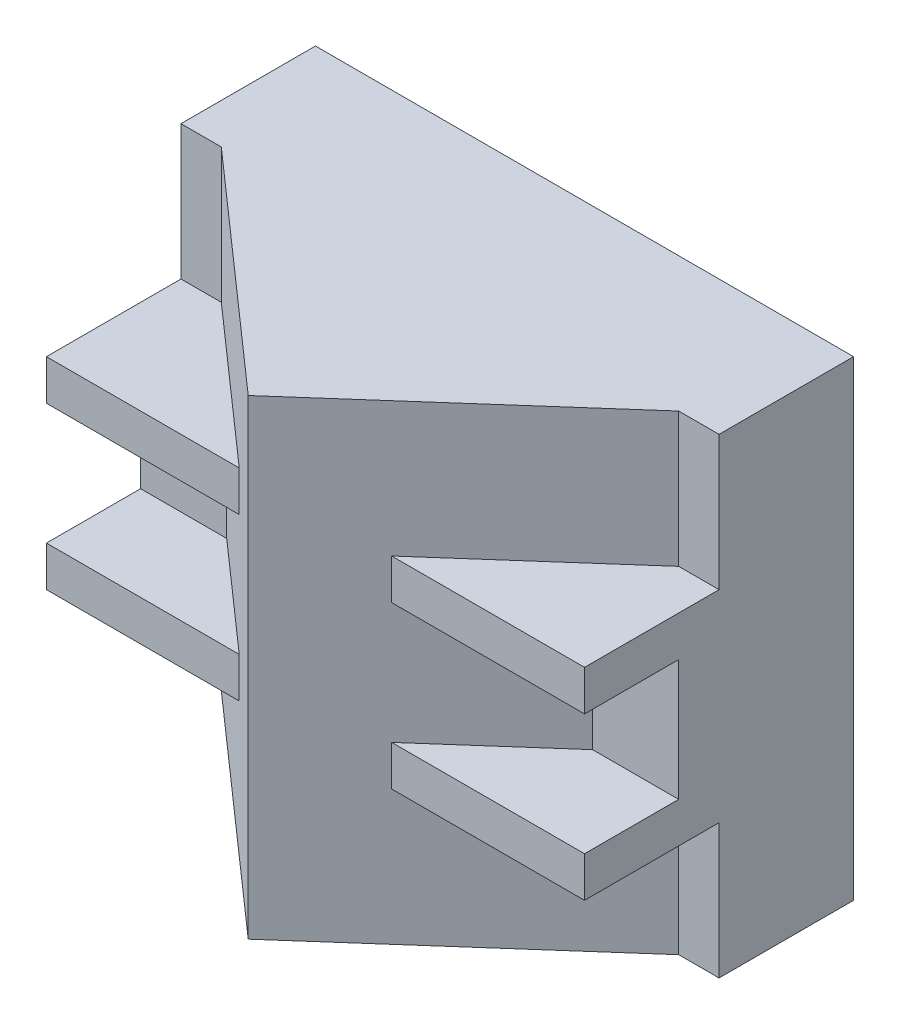
ISO-10303-21;
HEADER;
FILE_DESCRIPTION(('STEP AP214'),'2;1');
FILE_NAME('part.step','',(''),(''),'','','');
FILE_SCHEMA(('AUTOMOTIVE_DESIGN { 1 0 10303 214 1 1 1 1 }'));
ENDSEC;
DATA;
#1=APPLICATION_CONTEXT('core data for automotive mechanical design processes');
#2=APPLICATION_PROTOCOL_DEFINITION('international standard','automotive_design',2000,#1);
#3=PRODUCT_CONTEXT('',#1,'mechanical');
#4=PRODUCT('Part','Part','',(#3));
#5=PRODUCT_RELATED_PRODUCT_CATEGORY('part','',(#4));
#6=PRODUCT_DEFINITION_FORMATION('','',#4);
#7=PRODUCT_DEFINITION_CONTEXT('part definition',#1,'design');
#8=PRODUCT_DEFINITION('design','',#6,#7);
#9=PRODUCT_DEFINITION_SHAPE('','',#8);
#10=(LENGTH_UNIT() NAMED_UNIT(*) SI_UNIT(.MILLI.,.METRE.));
#11=(NAMED_UNIT(*) PLANE_ANGLE_UNIT() SI_UNIT($,.RADIAN.));
#12=(NAMED_UNIT(*) SI_UNIT($,.STERADIAN.) SOLID_ANGLE_UNIT());
#13=UNCERTAINTY_MEASURE_WITH_UNIT(LENGTH_MEASURE(1.E-05),#10,'distance_accuracy_value','');
#14=(GEOMETRIC_REPRESENTATION_CONTEXT(3) GLOBAL_UNCERTAINTY_ASSIGNED_CONTEXT((#13)) GLOBAL_UNIT_ASSIGNED_CONTEXT((#10,
#11,#12)) REPRESENTATION_CONTEXT('',''));
#15=CARTESIAN_POINT('',(0.,0.,0.));
#16=DIRECTION('',(0.,0.,1.));
#17=DIRECTION('',(1.,0.,0.));
#18=AXIS2_PLACEMENT_3D('',#15,#16,#17);
#19=CARTESIAN_POINT('',(0.,0.,0.));
#20=DIRECTION('',(0.,0.,-1.));
#21=DIRECTION('',(-1.,0.,0.));
#22=AXIS2_PLACEMENT_3D('',#19,#20,#21);
#23=PLANE('',#22);
#24=DIRECTION('',(1.,0.,0.));
#25=VECTOR('',#24,1.);
#26=CARTESIAN_POINT('',(0.,50.,0.));
#27=LINE('',#26,#25);
#28=CARTESIAN_POINT('',(0.,50.,0.));
#29=VERTEX_POINT('',#28);
#30=CARTESIAN_POINT('',(15.,50.,0.));
#31=VERTEX_POINT('',#30);
#32=EDGE_CURVE('E61',#29,#31,#27,.T.);
#33=ORIENTED_EDGE('',*,*,#32,.F.);
#34=DIRECTION('',(0.,-1.,0.));
#35=VECTOR('',#34,1.);
#36=CARTESIAN_POINT('',(0.,0.,0.));
#37=LINE('',#36,#35);
#38=CARTESIAN_POINT('',(0.,0.,0.));
#39=VERTEX_POINT('',#38);
#40=EDGE_CURVE('E311',#29,#39,#37,.T.);
#41=ORIENTED_EDGE('',*,*,#40,.T.);
#42=DIRECTION('',(1.,0.,0.));
#43=VECTOR('',#42,1.);
#44=CARTESIAN_POINT('',(0.,0.,0.));
#45=LINE('',#44,#43);
#46=CARTESIAN_POINT('',(15.,0.,0.));
#47=VERTEX_POINT('',#46);
#48=EDGE_CURVE('E336',#39,#47,#45,.T.);
#49=ORIENTED_EDGE('',*,*,#48,.T.);
#50=DIRECTION('',(0.,-1.,0.));
#51=VECTOR('',#50,1.);
#52=CARTESIAN_POINT('',(15.,175.,0.));
#53=LINE('',#52,#51);
#54=EDGE_CURVE('E318',#31,#47,#53,.T.);
#55=ORIENTED_EDGE('',*,*,#54,.F.);
#56=EDGE_LOOP('',(#33,#41,#49,#55));
#57=FACE_BOUND('',#56,.T.);
#58=ADVANCED_FACE('F50',(#57),#23,.F.);
#59=CARTESIAN_POINT('',(185.,50.,0.));
#60=VERTEX_POINT('',#59);
#61=CARTESIAN_POINT('',(200.,50.,0.));
#62=VERTEX_POINT('',#61);
#63=EDGE_CURVE('E277',#60,#62,#27,.T.);
#64=ORIENTED_EDGE('',*,*,#63,.F.);
#65=DIRECTION('',(0.,-1.,0.));
#66=VECTOR('',#65,1.);
#67=CARTESIAN_POINT('',(185.,175.,0.));
#68=LINE('',#67,#66);
#69=CARTESIAN_POINT('',(185.,0.,0.));
#70=VERTEX_POINT('',#69);
#71=EDGE_CURVE('E314',#60,#70,#68,.T.);
#72=ORIENTED_EDGE('',*,*,#71,.T.);
#73=CARTESIAN_POINT('',(200.,0.,0.));
#74=VERTEX_POINT('',#73);
#75=EDGE_CURVE('E339',#70,#74,#45,.T.);
#76=ORIENTED_EDGE('',*,*,#75,.T.);
#77=DIRECTION('',(0.,1.,0.));
#78=VECTOR('',#77,1.);
#79=CARTESIAN_POINT('',(200.,0.,0.));
#80=LINE('',#79,#78);
#81=EDGE_CURVE('E342',#74,#62,#80,.T.);
#82=ORIENTED_EDGE('',*,*,#81,.T.);
#83=EDGE_LOOP('',(#64,#72,#76,#82));
#84=FACE_BOUND('',#83,.T.);
#85=ADVANCED_FACE('F410',(#84),#23,.F.);
#86=CARTESIAN_POINT('',(0.,175.,0.));
#87=VERTEX_POINT('',#86);
#88=CARTESIAN_POINT('',(0.,125.,0.));
#89=VERTEX_POINT('',#88);
#90=EDGE_CURVE('E68',#87,#89,#37,.T.);
#91=ORIENTED_EDGE('',*,*,#90,.T.);
#92=DIRECTION('',(1.,0.,0.));
#93=VECTOR('',#92,1.);
#94=CARTESIAN_POINT('',(0.,125.,0.));
#95=LINE('',#94,#93);
#96=CARTESIAN_POINT('',(15.,125.,0.));
#97=VERTEX_POINT('',#96);
#98=EDGE_CURVE('E275',#89,#97,#95,.T.);
#99=ORIENTED_EDGE('',*,*,#98,.T.);
#100=CARTESIAN_POINT('',(15.,175.,0.));
#101=VERTEX_POINT('',#100);
#102=EDGE_CURVE('E312',#101,#97,#53,.T.);
#103=ORIENTED_EDGE('',*,*,#102,.F.);
#104=DIRECTION('',(-1.,0.,0.));
#105=VECTOR('',#104,1.);
#106=CARTESIAN_POINT('',(0.,175.,0.));
#107=LINE('',#106,#105);
#108=EDGE_CURVE('E345',#101,#87,#107,.T.);
#109=ORIENTED_EDGE('',*,*,#108,.T.);
#110=EDGE_LOOP('',(#91,#99,#103,#109));
#111=FACE_BOUND('',#110,.T.);
#112=ADVANCED_FACE('F381',(#111),#23,.F.);
#113=CARTESIAN_POINT('',(0.,0.,-50.));
#114=DIRECTION('',(-1.,0.,0.));
#115=DIRECTION('',(0.,0.,1.));
#116=AXIS2_PLACEMENT_3D('',#113,#114,#115);
#117=PLANE('',#116);
#118=ORIENTED_EDGE('',*,*,#90,.F.);
#119=DIRECTION('',(0.,0.,1.));
#120=VECTOR('',#119,1.);
#121=CARTESIAN_POINT('',(0.,175.,-50.));
#122=LINE('',#121,#120);
#123=CARTESIAN_POINT('',(0.,175.,-50.));
#124=VERTEX_POINT('',#123);
#125=EDGE_CURVE('E347',#124,#87,#122,.T.);
#126=ORIENTED_EDGE('',*,*,#125,.F.);
#127=DIRECTION('',(0.,-1.,0.));
#128=VECTOR('',#127,1.);
#129=CARTESIAN_POINT('',(0.,0.,-50.));
#130=LINE('',#129,#128);
#131=CARTESIAN_POINT('',(0.,0.,-50.));
#132=VERTEX_POINT('',#131);
#133=EDGE_CURVE('E321',#124,#132,#130,.T.);
#134=ORIENTED_EDGE('',*,*,#133,.T.);
#135=DIRECTION('',(0.,0.,1.));
#136=VECTOR('',#135,1.);
#137=CARTESIAN_POINT('',(0.,0.,-50.));
#138=LINE('',#137,#136);
#139=EDGE_CURVE('E331',#132,#39,#138,.T.);
#140=ORIENTED_EDGE('',*,*,#139,.T.);
#141=ORIENTED_EDGE('',*,*,#40,.F.);
#142=DIRECTION('',(0.,0.,1.));
#143=VECTOR('',#142,1.);
#144=CARTESIAN_POINT('',(0.,50.,0.));
#145=LINE('',#144,#143);
#146=CARTESIAN_POINT('',(0.,50.,50.));
#147=VERTEX_POINT('',#146);
#148=EDGE_CURVE('E231',#29,#147,#145,.T.);
#149=ORIENTED_EDGE('',*,*,#148,.T.);
#150=DIRECTION('',(0.,1.,0.));
#151=VECTOR('',#150,1.);
#152=CARTESIAN_POINT('',(0.,0.,50.));
#153=LINE('',#152,#151);
#154=CARTESIAN_POINT('',(0.,65.,50.));
#155=VERTEX_POINT('',#154);
#156=EDGE_CURVE('E208',#147,#155,#153,.T.);
#157=ORIENTED_EDGE('',*,*,#156,.T.);
#158=DIRECTION('',(0.,0.,-1.));
#159=VECTOR('',#158,1.);
#160=CARTESIAN_POINT('',(0.,65.,0.));
#161=LINE('',#160,#159);
#162=CARTESIAN_POINT('',(0.,65.,15.));
#163=VERTEX_POINT('',#162);
#164=EDGE_CURVE('E203',#155,#163,#161,.T.);
#165=ORIENTED_EDGE('',*,*,#164,.T.);
#166=DIRECTION('',(0.,1.,0.));
#167=VECTOR('',#166,1.);
#168=CARTESIAN_POINT('',(0.,0.,15.));
#169=LINE('',#168,#167);
#170=CARTESIAN_POINT('',(0.,110.,15.));
#171=VERTEX_POINT('',#170);
#172=EDGE_CURVE('E202',#163,#171,#169,.T.);
#173=ORIENTED_EDGE('',*,*,#172,.T.);
#174=DIRECTION('',(0.,0.,-1.));
#175=VECTOR('',#174,1.);
#176=CARTESIAN_POINT('',(0.,110.,0.));
#177=LINE('',#176,#175);
#178=CARTESIAN_POINT('',(0.,110.,50.));
#179=VERTEX_POINT('',#178);
#180=EDGE_CURVE('E241',#179,#171,#177,.T.);
#181=ORIENTED_EDGE('',*,*,#180,.F.);
#182=DIRECTION('',(0.,-1.,0.));
#183=VECTOR('',#182,1.);
#184=CARTESIAN_POINT('',(0.,0.,50.));
#185=LINE('',#184,#183);
#186=CARTESIAN_POINT('',(0.,125.,50.));
#187=VERTEX_POINT('',#186);
#188=EDGE_CURVE('E239',#187,#179,#185,.T.);
#189=ORIENTED_EDGE('',*,*,#188,.F.);
#190=DIRECTION('',(0.,0.,1.));
#191=VECTOR('',#190,1.);
#192=CARTESIAN_POINT('',(0.,125.,0.));
#193=LINE('',#192,#191);
#194=EDGE_CURVE('E237',#89,#187,#193,.T.);
#195=ORIENTED_EDGE('',*,*,#194,.F.);
#196=EDGE_LOOP('',(#118,#126,#134,#140,#141,#149,#157,#165,#173,#181,#189,#195));
#197=FACE_BOUND('',#196,.T.);
#198=ADVANCED_FACE('F47',(#197),#117,.T.);
#199=CARTESIAN_POINT('',(0.,175.,-50.));
#200=DIRECTION('',(0.,1.,0.));
#201=DIRECTION('',(0.,0.,1.));
#202=AXIS2_PLACEMENT_3D('',#199,#200,#201);
#203=PLANE('',#202);
#204=CARTESIAN_POINT('',(200.,175.,0.));
#205=VERTEX_POINT('',#204);
#206=CARTESIAN_POINT('',(185.,175.,0.));
#207=VERTEX_POINT('',#206);
#208=EDGE_CURVE('E324',#205,#207,#107,.T.);
#209=ORIENTED_EDGE('',*,*,#208,.F.);
#210=DIRECTION('',(0.,0.,1.));
#211=VECTOR('',#210,1.);
#212=CARTESIAN_POINT('',(200.,175.,-50.));
#213=LINE('',#212,#211);
#214=CARTESIAN_POINT('',(200.,175.,-50.));
#215=VERTEX_POINT('',#214);
#216=EDGE_CURVE('E349',#215,#205,#213,.T.);
#217=ORIENTED_EDGE('',*,*,#216,.F.);
#218=DIRECTION('',(-1.,0.,0.));
#219=VECTOR('',#218,1.);
#220=CARTESIAN_POINT('',(0.,175.,-50.));
#221=LINE('',#220,#219);
#222=EDGE_CURVE('E332',#215,#124,#221,.T.);
#223=ORIENTED_EDGE('',*,*,#222,.T.);
#224=ORIENTED_EDGE('',*,*,#125,.T.);
#225=ORIENTED_EDGE('',*,*,#108,.F.);
#226=DIRECTION('',(0.749837855365093,0.,0.661621637086846));
#227=VECTOR('',#226,1.);
#228=CARTESIAN_POINT('',(6.56614785992218,175.,-7.44163424124514));
#229=LINE('',#228,#227);
#230=CARTESIAN_POINT('',(100.,175.,75.));
#231=VERTEX_POINT('',#230);
#232=EDGE_CURVE('E305',#101,#231,#229,.T.);
#233=ORIENTED_EDGE('',*,*,#232,.T.);
#234=DIRECTION('',(0.749837855365093,0.,-0.661621637086846));
#235=VECTOR('',#234,1.);
#236=CARTESIAN_POINT('',(80.9824902723735,175.,91.7801556420233));
#237=LINE('',#236,#235);
#238=EDGE_CURVE('E302',#231,#207,#237,.T.);
#239=ORIENTED_EDGE('',*,*,#238,.T.);
#240=EDGE_LOOP('',(#209,#217,#223,#224,#225,#233,#239));
#241=FACE_BOUND('',#240,.T.);
#242=ADVANCED_FACE('F390',(#241),#203,.T.);
#243=CARTESIAN_POINT('',(200.,0.,-50.));
#244=DIRECTION('',(1.,0.,0.));
#245=DIRECTION('',(0.,0.,-1.));
#246=AXIS2_PLACEMENT_3D('',#243,#244,#245);
#247=PLANE('',#246);
#248=ORIENTED_EDGE('',*,*,#81,.F.);
#249=DIRECTION('',(0.,0.,1.));
#250=VECTOR('',#249,1.);
#251=CARTESIAN_POINT('',(200.,0.,-50.));
#252=LINE('',#251,#250);
#253=CARTESIAN_POINT('',(200.,0.,-50.));
#254=VERTEX_POINT('',#253);
#255=EDGE_CURVE('E351',#254,#74,#252,.T.);
#256=ORIENTED_EDGE('',*,*,#255,.F.);
#257=DIRECTION('',(0.,1.,0.));
#258=VECTOR('',#257,1.);
#259=CARTESIAN_POINT('',(200.,0.,-50.));
#260=LINE('',#259,#258);
#261=EDGE_CURVE('E327',#254,#215,#260,.T.);
#262=ORIENTED_EDGE('',*,*,#261,.T.);
#263=ORIENTED_EDGE('',*,*,#216,.T.);
#264=CARTESIAN_POINT('',(200.,125.,0.));
#265=VERTEX_POINT('',#264);
#266=EDGE_CURVE('E337',#265,#205,#80,.T.);
#267=ORIENTED_EDGE('',*,*,#266,.F.);
#268=DIRECTION('',(0.,0.,1.));
#269=VECTOR('',#268,1.);
#270=CARTESIAN_POINT('',(200.,125.,0.));
#271=LINE('',#270,#269);
#272=CARTESIAN_POINT('',(200.,125.,50.));
#273=VERTEX_POINT('',#272);
#274=EDGE_CURVE('E258',#265,#273,#271,.T.);
#275=ORIENTED_EDGE('',*,*,#274,.T.);
#276=DIRECTION('',(0.,-1.,0.));
#277=VECTOR('',#276,1.);
#278=CARTESIAN_POINT('',(200.,0.,50.));
#279=LINE('',#278,#277);
#280=CARTESIAN_POINT('',(200.,110.,50.));
#281=VERTEX_POINT('',#280);
#282=EDGE_CURVE('E227',#273,#281,#279,.T.);
#283=ORIENTED_EDGE('',*,*,#282,.T.);
#284=DIRECTION('',(0.,0.,-1.));
#285=VECTOR('',#284,1.);
#286=CARTESIAN_POINT('',(200.,110.,0.));
#287=LINE('',#286,#285);
#288=CARTESIAN_POINT('',(200.,110.,15.));
#289=VERTEX_POINT('',#288);
#290=EDGE_CURVE('E226',#281,#289,#287,.T.);
#291=ORIENTED_EDGE('',*,*,#290,.T.);
#292=DIRECTION('',(0.,1.,0.));
#293=VECTOR('',#292,1.);
#294=CARTESIAN_POINT('',(200.,0.,15.));
#295=LINE('',#294,#293);
#296=CARTESIAN_POINT('',(200.,65.,15.));
#297=VERTEX_POINT('',#296);
#298=EDGE_CURVE('E243',#297,#289,#295,.T.);
#299=ORIENTED_EDGE('',*,*,#298,.F.);
#300=DIRECTION('',(0.,0.,-1.));
#301=VECTOR('',#300,1.);
#302=CARTESIAN_POINT('',(200.,65.,0.));
#303=LINE('',#302,#301);
#304=CARTESIAN_POINT('',(200.,65.,50.));
#305=VERTEX_POINT('',#304);
#306=EDGE_CURVE('E249',#305,#297,#303,.T.);
#307=ORIENTED_EDGE('',*,*,#306,.F.);
#308=DIRECTION('',(0.,1.,0.));
#309=VECTOR('',#308,1.);
#310=CARTESIAN_POINT('',(200.,0.,50.));
#311=LINE('',#310,#309);
#312=CARTESIAN_POINT('',(200.,50.,50.));
#313=VERTEX_POINT('',#312);
#314=EDGE_CURVE('E248',#313,#305,#311,.T.);
#315=ORIENTED_EDGE('',*,*,#314,.F.);
#316=DIRECTION('',(0.,0.,1.));
#317=VECTOR('',#316,1.);
#318=CARTESIAN_POINT('',(200.,50.,0.));
#319=LINE('',#318,#317);
#320=EDGE_CURVE('E251',#62,#313,#319,.T.);
#321=ORIENTED_EDGE('',*,*,#320,.F.);
#322=EDGE_LOOP('',(#248,#256,#262,#263,#267,#275,#283,#291,#299,#307,#315,#321));
#323=FACE_BOUND('',#322,.T.);
#324=ADVANCED_FACE('F432',(#323),#247,.T.);
#325=CARTESIAN_POINT('',(0.,0.,-50.));
#326=DIRECTION('',(0.,-1.,0.));
#327=DIRECTION('',(0.,0.,-1.));
#328=AXIS2_PLACEMENT_3D('',#325,#326,#327);
#329=PLANE('',#328);
#330=ORIENTED_EDGE('',*,*,#48,.F.);
#331=ORIENTED_EDGE('',*,*,#139,.F.);
#332=DIRECTION('',(1.,0.,0.));
#333=VECTOR('',#332,1.);
#334=CARTESIAN_POINT('',(0.,0.,-50.));
#335=LINE('',#334,#333);
#336=EDGE_CURVE('E322',#132,#254,#335,.T.);
#337=ORIENTED_EDGE('',*,*,#336,.T.);
#338=ORIENTED_EDGE('',*,*,#255,.T.);
#339=ORIENTED_EDGE('',*,*,#75,.F.);
#340=DIRECTION('',(0.749837855365093,0.,-0.661621637086846));
#341=VECTOR('',#340,1.);
#342=CARTESIAN_POINT('',(80.9824902723735,0.,91.7801556420233));
#343=LINE('',#342,#341);
#344=CARTESIAN_POINT('',(100.,0.,75.));
#345=VERTEX_POINT('',#344);
#346=EDGE_CURVE('E297',#345,#70,#343,.T.);
#347=ORIENTED_EDGE('',*,*,#346,.F.);
#348=DIRECTION('',(0.749837855365093,0.,0.661621637086846));
#349=VECTOR('',#348,1.);
#350=CARTESIAN_POINT('',(6.56614785992218,0.,-7.44163424124514));
#351=LINE('',#350,#349);
#352=EDGE_CURVE('E301',#47,#345,#351,.T.);
#353=ORIENTED_EDGE('',*,*,#352,.F.);
#354=EDGE_LOOP('',(#330,#331,#337,#338,#339,#347,#353));
#355=FACE_BOUND('',#354,.T.);
#356=ADVANCED_FACE('F399',(#355),#329,.T.);
#357=CARTESIAN_POINT('',(0.,0.,-50.));
#358=DIRECTION('',(0.,0.,-1.));
#359=DIRECTION('',(-1.,0.,0.));
#360=AXIS2_PLACEMENT_3D('',#357,#358,#359);
#361=PLANE('',#360);
#362=ORIENTED_EDGE('',*,*,#133,.F.);
#363=ORIENTED_EDGE('',*,*,#222,.F.);
#364=ORIENTED_EDGE('',*,*,#261,.F.);
#365=ORIENTED_EDGE('',*,*,#336,.F.);
#366=EDGE_LOOP('',(#362,#363,#364,#365));
#367=FACE_BOUND('',#366,.T.);
#368=ADVANCED_FACE('F395',(#367),#361,.T.);
#369=CARTESIAN_POINT('',(185.,125.,0.));
#370=VERTEX_POINT('',#369);
#371=EDGE_CURVE('E309',#207,#370,#68,.T.);
#372=ORIENTED_EDGE('',*,*,#371,.T.);
#373=EDGE_CURVE('E273',#370,#265,#95,.T.);
#374=ORIENTED_EDGE('',*,*,#373,.T.);
#375=ORIENTED_EDGE('',*,*,#266,.T.);
#376=ORIENTED_EDGE('',*,*,#208,.T.);
#377=EDGE_LOOP('',(#372,#374,#375,#376));
#378=FACE_BOUND('',#377,.T.);
#379=ADVANCED_FACE('F407',(#378),#23,.F.);
#380=CARTESIAN_POINT('',(80.9824902723735,175.,91.7801556420233));
#381=DIRECTION('',(-0.661621637086846,0.,-0.749837855365092));
#382=DIRECTION('',(-0.749837855365093,0.,0.661621637086846));
#383=AXIS2_PLACEMENT_3D('',#380,#381,#382);
#384=PLANE('',#383);
#385=DIRECTION('',(0.,1.,0.));
#386=VECTOR('',#385,1.);
#387=CARTESIAN_POINT('',(128.333333333333,175.,50.));
#388=LINE('',#387,#386);
#389=CARTESIAN_POINT('',(128.333333333333,110.,50.));
#390=VERTEX_POINT('',#389);
#391=CARTESIAN_POINT('',(128.333333333333,125.,50.));
#392=VERTEX_POINT('',#391);
#393=EDGE_CURVE('E291',#390,#392,#388,.T.);
#394=ORIENTED_EDGE('',*,*,#393,.T.);
#395=DIRECTION('',(0.749837855365093,0.,-0.661621637086846));
#396=VECTOR('',#395,1.);
#397=CARTESIAN_POINT('',(80.9824902723735,125.,91.7801556420233));
#398=LINE('',#397,#396);
#399=EDGE_CURVE('E292',#392,#370,#398,.T.);
#400=ORIENTED_EDGE('',*,*,#399,.T.);
#401=ORIENTED_EDGE('',*,*,#371,.F.);
#402=ORIENTED_EDGE('',*,*,#238,.F.);
#403=DIRECTION('',(0.,-1.,0.));
#404=VECTOR('',#403,1.);
#405=CARTESIAN_POINT('',(100.,175.,75.));
#406=LINE('',#405,#404);
#407=EDGE_CURVE('E308',#231,#345,#406,.T.);
#408=ORIENTED_EDGE('',*,*,#407,.T.);
#409=ORIENTED_EDGE('',*,*,#346,.T.);
#410=ORIENTED_EDGE('',*,*,#71,.F.);
#411=DIRECTION('',(0.749837855365093,0.,-0.661621637086846));
#412=VECTOR('',#411,1.);
#413=CARTESIAN_POINT('',(80.9824902723735,50.,91.7801556420233));
#414=LINE('',#413,#412);
#415=CARTESIAN_POINT('',(128.333333333333,50.,50.));
#416=VERTEX_POINT('',#415);
#417=EDGE_CURVE('E290',#416,#60,#414,.T.);
#418=ORIENTED_EDGE('',*,*,#417,.F.);
#419=DIRECTION('',(0.,-1.,0.));
#420=VECTOR('',#419,1.);
#421=CARTESIAN_POINT('',(128.333333333333,175.,50.));
#422=LINE('',#421,#420);
#423=CARTESIAN_POINT('',(128.333333333333,65.,50.));
#424=VERTEX_POINT('',#423);
#425=EDGE_CURVE('E282',#424,#416,#422,.T.);
#426=ORIENTED_EDGE('',*,*,#425,.F.);
#427=DIRECTION('',(-0.749837855365093,0.,0.661621637086846));
#428=VECTOR('',#427,1.);
#429=CARTESIAN_POINT('',(80.9824902723735,65.,91.7801556420233));
#430=LINE('',#429,#428);
#431=CARTESIAN_POINT('',(168.,65.,15.));
#432=VERTEX_POINT('',#431);
#433=EDGE_CURVE('E265',#432,#424,#430,.T.);
#434=ORIENTED_EDGE('',*,*,#433,.F.);
#435=DIRECTION('',(0.,-1.,0.));
#436=VECTOR('',#435,1.);
#437=CARTESIAN_POINT('',(168.,175.,15.));
#438=LINE('',#437,#436);
#439=CARTESIAN_POINT('',(168.,110.,15.));
#440=VERTEX_POINT('',#439);
#441=EDGE_CURVE('E296',#440,#432,#438,.T.);
#442=ORIENTED_EDGE('',*,*,#441,.F.);
#443=DIRECTION('',(-0.749837855365093,0.,0.661621637086846));
#444=VECTOR('',#443,1.);
#445=CARTESIAN_POINT('',(80.9824902723735,110.,91.7801556420233));
#446=LINE('',#445,#444);
#447=EDGE_CURVE('E293',#440,#390,#446,.T.);
#448=ORIENTED_EDGE('',*,*,#447,.T.);
#449=EDGE_LOOP('',(#394,#400,#401,#402,#408,#409,#410,#418,#426,#434,#442,#448));
#450=FACE_BOUND('',#449,.T.);
#451=ADVANCED_FACE('F416',(#450),#384,.F.);
#452=CARTESIAN_POINT('',(6.56614785992218,175.,-7.44163424124514));
#453=DIRECTION('',(0.661621637086846,0.,-0.749837855365093));
#454=DIRECTION('',(-0.749837855365093,0.,-0.661621637086846));
#455=AXIS2_PLACEMENT_3D('',#452,#453,#454);
#456=PLANE('',#455);
#457=ORIENTED_EDGE('',*,*,#102,.T.);
#458=DIRECTION('',(0.749837855365093,0.,0.661621637086846));
#459=VECTOR('',#458,1.);
#460=CARTESIAN_POINT('',(6.56614785992218,125.,-7.44163424124514));
#461=LINE('',#460,#459);
#462=CARTESIAN_POINT('',(71.6666666666667,125.,50.));
#463=VERTEX_POINT('',#462);
#464=EDGE_CURVE('E11',#97,#463,#461,.T.);
#465=ORIENTED_EDGE('',*,*,#464,.T.);
#466=DIRECTION('',(0.,-1.,0.));
#467=VECTOR('',#466,1.);
#468=CARTESIAN_POINT('',(71.6666666666667,175.,50.));
#469=LINE('',#468,#467);
#470=CARTESIAN_POINT('',(71.6666666666667,110.,50.));
#471=VERTEX_POINT('',#470);
#472=EDGE_CURVE('E54',#463,#471,#469,.T.);
#473=ORIENTED_EDGE('',*,*,#472,.T.);
#474=DIRECTION('',(-0.749837855365093,0.,-0.661621637086846));
#475=VECTOR('',#474,1.);
#476=CARTESIAN_POINT('',(6.56614785992218,110.,-7.44163424124514));
#477=LINE('',#476,#475);
#478=CARTESIAN_POINT('',(32.,110.,15.));
#479=VERTEX_POINT('',#478);
#480=EDGE_CURVE('E368',#471,#479,#477,.T.);
#481=ORIENTED_EDGE('',*,*,#480,.T.);
#482=DIRECTION('',(0.,1.,0.));
#483=VECTOR('',#482,1.);
#484=CARTESIAN_POINT('',(32.,175.,15.));
#485=LINE('',#484,#483);
#486=CARTESIAN_POINT('',(32.,65.,15.));
#487=VERTEX_POINT('',#486);
#488=EDGE_CURVE('E365',#487,#479,#485,.T.);
#489=ORIENTED_EDGE('',*,*,#488,.F.);
#490=DIRECTION('',(-0.749837855365093,0.,-0.661621637086846));
#491=VECTOR('',#490,1.);
#492=CARTESIAN_POINT('',(6.56614785992218,65.,-7.44163424124514));
#493=LINE('',#492,#491);
#494=CARTESIAN_POINT('',(71.6666666666667,65.,50.));
#495=VERTEX_POINT('',#494);
#496=EDGE_CURVE('E220',#495,#487,#493,.T.);
#497=ORIENTED_EDGE('',*,*,#496,.F.);
#498=DIRECTION('',(0.,1.,0.));
#499=VECTOR('',#498,1.);
#500=CARTESIAN_POINT('',(71.6666666666667,175.,50.));
#501=LINE('',#500,#499);
#502=CARTESIAN_POINT('',(71.6666666666667,50.,50.));
#503=VERTEX_POINT('',#502);
#504=EDGE_CURVE('E360',#503,#495,#501,.T.);
#505=ORIENTED_EDGE('',*,*,#504,.F.);
#506=DIRECTION('',(0.749837855365093,0.,0.661621637086846));
#507=VECTOR('',#506,1.);
#508=CARTESIAN_POINT('',(6.56614785992218,50.,-7.44163424124514));
#509=LINE('',#508,#507);
#510=EDGE_CURVE('E363',#31,#503,#509,.T.);
#511=ORIENTED_EDGE('',*,*,#510,.F.);
#512=ORIENTED_EDGE('',*,*,#54,.T.);
#513=ORIENTED_EDGE('',*,*,#352,.T.);
#514=ORIENTED_EDGE('',*,*,#407,.F.);
#515=ORIENTED_EDGE('',*,*,#232,.F.);
#516=EDGE_LOOP('',(#457,#465,#473,#481,#489,#497,#505,#511,#512,#513,#514,#515));
#517=FACE_BOUND('',#516,.T.);
#518=ADVANCED_FACE('F367',(#517),#456,.F.);
#519=CARTESIAN_POINT('',(0.,125.,0.));
#520=DIRECTION('',(0.,1.,0.));
#521=DIRECTION('',(0.,0.,1.));
#522=AXIS2_PLACEMENT_3D('',#519,#520,#521);
#523=PLANE('',#522);
#524=ORIENTED_EDGE('',*,*,#464,.F.);
#525=ORIENTED_EDGE('',*,*,#98,.F.);
#526=ORIENTED_EDGE('',*,*,#194,.T.);
#527=DIRECTION('',(1.,0.,0.));
#528=VECTOR('',#527,1.);
#529=CARTESIAN_POINT('',(0.,125.,50.));
#530=LINE('',#529,#528);
#531=EDGE_CURVE('E268',#187,#463,#530,.T.);
#532=ORIENTED_EDGE('',*,*,#531,.T.);
#533=EDGE_LOOP('',(#524,#525,#526,#532));
#534=FACE_BOUND('',#533,.T.);
#535=ADVANCED_FACE('F377',(#534),#523,.T.);
#536=CARTESIAN_POINT('',(0.,0.,50.));
#537=DIRECTION('',(0.,0.,1.));
#538=DIRECTION('',(1.,0.,0.));
#539=AXIS2_PLACEMENT_3D('',#536,#537,#538);
#540=PLANE('',#539);
#541=ORIENTED_EDGE('',*,*,#472,.F.);
#542=ORIENTED_EDGE('',*,*,#531,.F.);
#543=ORIENTED_EDGE('',*,*,#188,.T.);
#544=DIRECTION('',(1.,0.,0.));
#545=VECTOR('',#544,1.);
#546=CARTESIAN_POINT('',(0.,110.,50.));
#547=LINE('',#546,#545);
#548=EDGE_CURVE('E262',#179,#471,#547,.T.);
#549=ORIENTED_EDGE('',*,*,#548,.T.);
#550=EDGE_LOOP('',(#541,#542,#543,#549));
#551=FACE_BOUND('',#550,.T.);
#552=ADVANCED_FACE('F374',(#551),#540,.T.);
#553=CARTESIAN_POINT('',(0.,110.,0.));
#554=DIRECTION('',(0.,-1.,0.));
#555=DIRECTION('',(0.,0.,-1.));
#556=AXIS2_PLACEMENT_3D('',#553,#554,#555);
#557=PLANE('',#556);
#558=ORIENTED_EDGE('',*,*,#480,.F.);
#559=ORIENTED_EDGE('',*,*,#548,.F.);
#560=ORIENTED_EDGE('',*,*,#180,.T.);
#561=DIRECTION('',(1.,0.,0.));
#562=VECTOR('',#561,1.);
#563=CARTESIAN_POINT('',(0.,110.,15.));
#564=LINE('',#563,#562);
#565=EDGE_CURVE('E223',#171,#479,#564,.T.);
#566=ORIENTED_EDGE('',*,*,#565,.T.);
#567=EDGE_LOOP('',(#558,#559,#560,#566));
#568=FACE_BOUND('',#567,.T.);
#569=ADVANCED_FACE('F372',(#568),#557,.T.);
#570=CARTESIAN_POINT('',(0.,65.,0.));
#571=DIRECTION('',(0.,-1.,0.));
#572=DIRECTION('',(0.,0.,-1.));
#573=AXIS2_PLACEMENT_3D('',#570,#571,#572);
#574=PLANE('',#573);
#575=DIRECTION('',(1.,0.,0.));
#576=VECTOR('',#575,1.);
#577=CARTESIAN_POINT('',(0.,65.,50.));
#578=LINE('',#577,#576);
#579=EDGE_CURVE('E284',#155,#495,#578,.T.);
#580=ORIENTED_EDGE('',*,*,#579,.T.);
#581=ORIENTED_EDGE('',*,*,#496,.T.);
#582=DIRECTION('',(1.,0.,0.));
#583=VECTOR('',#582,1.);
#584=CARTESIAN_POINT('',(0.,65.,15.));
#585=LINE('',#584,#583);
#586=EDGE_CURVE('E214',#163,#487,#585,.T.);
#587=ORIENTED_EDGE('',*,*,#586,.F.);
#588=ORIENTED_EDGE('',*,*,#164,.F.);
#589=EDGE_LOOP('',(#580,#581,#587,#588));
#590=FACE_BOUND('',#589,.T.);
#591=ADVANCED_FACE('F216',(#590),#574,.F.);
#592=CARTESIAN_POINT('',(0.,0.,50.));
#593=DIRECTION('',(0.,0.,-1.));
#594=DIRECTION('',(-1.,0.,0.));
#595=AXIS2_PLACEMENT_3D('',#592,#593,#594);
#596=PLANE('',#595);
#597=DIRECTION('',(1.,0.,0.));
#598=VECTOR('',#597,1.);
#599=CARTESIAN_POINT('',(0.,50.,50.));
#600=LINE('',#599,#598);
#601=EDGE_CURVE('E280',#147,#503,#600,.T.);
#602=ORIENTED_EDGE('',*,*,#601,.T.);
#603=ORIENTED_EDGE('',*,*,#504,.T.);
#604=ORIENTED_EDGE('',*,*,#579,.F.);
#605=ORIENTED_EDGE('',*,*,#156,.F.);
#606=EDGE_LOOP('',(#602,#603,#604,#605));
#607=FACE_BOUND('',#606,.T.);
#608=ADVANCED_FACE('F409',(#607),#596,.F.);
#609=CARTESIAN_POINT('',(0.,50.,0.));
#610=DIRECTION('',(0.,1.,0.));
#611=DIRECTION('',(0.,0.,1.));
#612=AXIS2_PLACEMENT_3D('',#609,#610,#611);
#613=PLANE('',#612);
#614=ORIENTED_EDGE('',*,*,#32,.T.);
#615=ORIENTED_EDGE('',*,*,#510,.T.);
#616=ORIENTED_EDGE('',*,*,#601,.F.);
#617=ORIENTED_EDGE('',*,*,#148,.F.);
#618=EDGE_LOOP('',(#614,#615,#616,#617));
#619=FACE_BOUND('',#618,.T.);
#620=ADVANCED_FACE('F404',(#619),#613,.F.);
#621=CARTESIAN_POINT('',(0.,0.,15.));
#622=DIRECTION('',(0.,0.,-1.));
#623=DIRECTION('',(-1.,0.,0.));
#624=AXIS2_PLACEMENT_3D('',#621,#622,#623);
#625=PLANE('',#624);
#626=ORIENTED_EDGE('',*,*,#586,.T.);
#627=ORIENTED_EDGE('',*,*,#488,.T.);
#628=ORIENTED_EDGE('',*,*,#565,.F.);
#629=ORIENTED_EDGE('',*,*,#172,.F.);
#630=EDGE_LOOP('',(#626,#627,#628,#629));
#631=FACE_BOUND('',#630,.T.);
#632=ADVANCED_FACE('F224',(#631),#625,.F.);
#633=EDGE_CURVE('E263',#440,#289,#564,.T.);
#634=ORIENTED_EDGE('',*,*,#633,.F.);
#635=ORIENTED_EDGE('',*,*,#441,.T.);
#636=EDGE_CURVE('E222',#432,#297,#585,.T.);
#637=ORIENTED_EDGE('',*,*,#636,.T.);
#638=ORIENTED_EDGE('',*,*,#298,.T.);
#639=EDGE_LOOP('',(#634,#635,#637,#638));
#640=FACE_BOUND('',#639,.T.);
#641=ADVANCED_FACE('F520',(#640),#625,.F.);
#642=ORIENTED_EDGE('',*,*,#447,.F.);
#643=ORIENTED_EDGE('',*,*,#633,.T.);
#644=ORIENTED_EDGE('',*,*,#290,.F.);
#645=EDGE_CURVE('E270',#390,#281,#547,.T.);
#646=ORIENTED_EDGE('',*,*,#645,.F.);
#647=EDGE_LOOP('',(#642,#643,#644,#646));
#648=FACE_BOUND('',#647,.T.);
#649=ADVANCED_FACE('F483',(#648),#557,.T.);
#650=ORIENTED_EDGE('',*,*,#393,.F.);
#651=ORIENTED_EDGE('',*,*,#645,.T.);
#652=ORIENTED_EDGE('',*,*,#282,.F.);
#653=EDGE_CURVE('E271',#392,#273,#530,.T.);
#654=ORIENTED_EDGE('',*,*,#653,.F.);
#655=EDGE_LOOP('',(#650,#651,#652,#654));
#656=FACE_BOUND('',#655,.T.);
#657=ADVANCED_FACE('F475',(#656),#540,.T.);
#658=ORIENTED_EDGE('',*,*,#399,.F.);
#659=ORIENTED_EDGE('',*,*,#653,.T.);
#660=ORIENTED_EDGE('',*,*,#274,.F.);
#661=ORIENTED_EDGE('',*,*,#373,.F.);
#662=EDGE_LOOP('',(#658,#659,#660,#661));
#663=FACE_BOUND('',#662,.T.);
#664=ADVANCED_FACE('F463',(#663),#523,.T.);
#665=EDGE_CURVE('E278',#416,#313,#600,.T.);
#666=ORIENTED_EDGE('',*,*,#665,.F.);
#667=ORIENTED_EDGE('',*,*,#417,.T.);
#668=ORIENTED_EDGE('',*,*,#63,.T.);
#669=ORIENTED_EDGE('',*,*,#320,.T.);
#670=EDGE_LOOP('',(#666,#667,#668,#669));
#671=FACE_BOUND('',#670,.T.);
#672=ADVANCED_FACE('F508',(#671),#613,.F.);
#673=EDGE_CURVE('E219',#424,#305,#578,.T.);
#674=ORIENTED_EDGE('',*,*,#673,.F.);
#675=ORIENTED_EDGE('',*,*,#425,.T.);
#676=ORIENTED_EDGE('',*,*,#665,.T.);
#677=ORIENTED_EDGE('',*,*,#314,.T.);
#678=EDGE_LOOP('',(#674,#675,#676,#677));
#679=FACE_BOUND('',#678,.T.);
#680=ADVANCED_FACE('F504',(#679),#596,.F.);
#681=ORIENTED_EDGE('',*,*,#636,.F.);
#682=ORIENTED_EDGE('',*,*,#433,.T.);
#683=ORIENTED_EDGE('',*,*,#673,.T.);
#684=ORIENTED_EDGE('',*,*,#306,.T.);
#685=EDGE_LOOP('',(#681,#682,#683,#684));
#686=FACE_BOUND('',#685,.T.);
#687=ADVANCED_FACE('F495',(#686),#574,.F.);
#688=CLOSED_SHELL('',(#58,#85,#112,#198,#242,#324,#356,#368,#379,#451,#518,#535,#552,#569,#591,
#608,#620,#632,#641,#649,#657,#664,#672,#680,#687));
#689=MANIFOLD_SOLID_BREP('B2',#688);
#690=ADVANCED_BREP_SHAPE_REPRESENTATION('',(#18,#689),#14);
#691=SHAPE_DEFINITION_REPRESENTATION(#9,#690);
ENDSEC;
END-ISO-10303-21;
